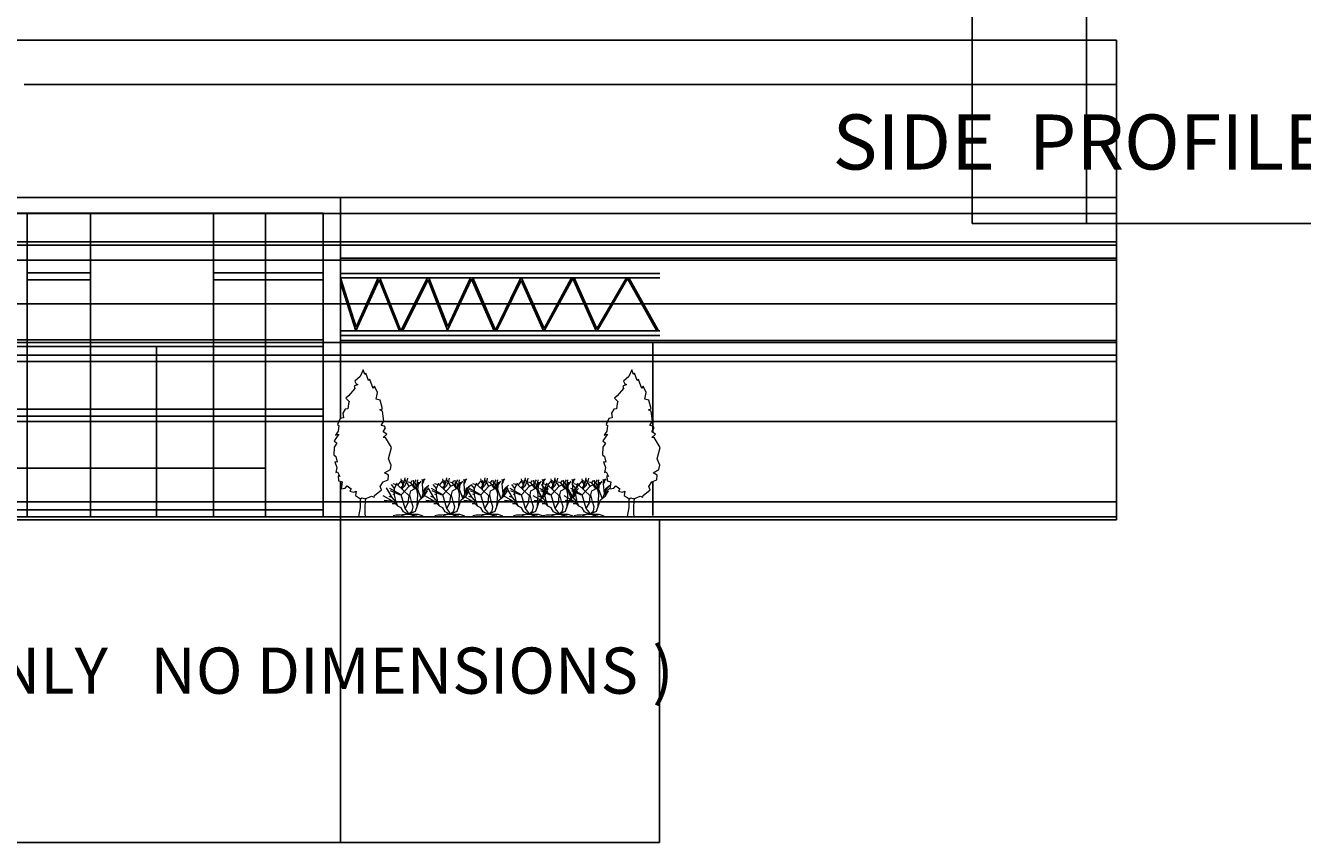
# Model space of a CAD drawing. Units: inches. Extents: x -32109 to 33221, y -19197 to 7608.
# Tile 14 of 25: x -741 to 10957, y -19197 to -11718. Entities that reach past the tile are written whole.
import ezdxf

# ---------------------------------------------------------------- set-up
doc = ezdxf.new("R2010")
doc.units = ezdxf.units.IN
doc.header["$MEASUREMENT"] = 0
for name, color, linetype, lineweight in [('A-ANNO-DIMS', 2, 'Continuous', 18), ('A-ANNO-TEXT', 7, 'Continuous', 25), ('A-ELEV', 7, 'Continuous', 25), ('L-PLNT', 3, 'Continuous', 13)]:
    doc.layers.add(name, color=color, linetype=linetype, lineweight=lineweight)
doc.styles.get("Standard").update_dxf_attribs({"font": 'arial.ttf'})
doc.dimstyles.get("Standard").update_dxf_attribs({"dimtxt": 0.18, "dimasz": 0.18, "dimexe": 0.18, "dimexo": 0.0625, "dimgap": 0.09, "dimtad": 0, "dimtih": 1, "dimtoh": 1, "dimdec": 4, "dimzin": 0, "dimdsep": 46, "dimtxsty": 'Standard', "dimcen": 0.09, "dimadec": 0, "dimazin": 0, "dimtfac": 1, "dimtdec": 4, "dimtofl": 0, "dimtmove": 0, "dimatfit": 3, "dimfxl": 1, "dimtolj": 1, "dimtzin": 0, "dimarcsym": 0})

# ---------------------------------------------------------------- blocks, each defined once
blk = doc.blocks.new('*U2')
blk.add_lwpolyline([(-2.75400000000036, 191.699), (-6.7800000000002, 182.8509999999996), (-13.68200000000024, 176.9529999999995), (-11.95600000000013, 173.2659999999996), (-9.655999999999949, 172.529), (-14.25700000000006, 170.317), (-13.68200000000024, 167.3679999999999), (-21.73300000000017, 157.7829999999999), (-25.1840000000002, 154.8340000000003), (-21.15800000000036, 150.4099999999998), (-21.73300000000017, 147.4609999999998), (-22.88400000000001, 140.8249999999998), (-26.33400000000029, 140.087), (-29.21000000000004, 134.9259999999995), (-28.63499999999977, 129.0279999999998), (-32.66100000000006, 128.2909999999997), (-36.11099999999988, 120.1799999999998), (-34.38599999999997, 118.7059999999997), (-35.53600000000006, 111.3329999999996), (-38.98700000000008, 106.1709999999998), (-34.38599999999997, 107.6459999999997), (-40.71199999999999, 98.79799999999977), (-37.26099999999997, 95.8489999999997), (-40.71199999999999, 90.68799999999965), (-41.28700000000026, 80.36599999999999), (-38.41200000000026, 78.154), (-36.68600000000015, 70.78099999999995), (-39.5619999999999, 71.51799999999957), (-37.26099999999997, 64.14499999999998), (-38.41200000000026, 57.50899999999956), (-36.11099999999988, 58.24699999999984), (-33.23599999999988, 52.3479999999995), (-35.53600000000006, 53.08599999999978), (-34.96100000000024, 46.44999999999981), (-30.36000000000013, 44.9749999999999), (-31.50999999999977, 36.1279999999997), (-26.33400000000029, 36.86499999999978), (-23.45900000000029, 39.81399999999985), (-18.28300000000036, 36.1279999999997), (-20.00800000000027, 33.17799999999988), (-14.83199999999988, 31.70399999999972), (-11.95600000000013, 33.17799999999988), (-12.53099999999995, 27.27999999999975), (-6.204999999999927, 22.85599999999977), (-3.9050000000002, 24.33099999999968), (0.1209999999996398, 22.85599999999977), (8.172999999999774, 26.54299999999967), (11.62399999999979, 25.06799999999976), (12.19900000000007, 27.27999999999975), (21.40000000000009, 34.6529999999998), (19.67500000000018, 39.07699999999977), (23.70099999999957, 44.9749999999999), (30.02700000000004, 47.92399999999997), (30.60199999999986, 53.82299999999986), (25.42599999999993, 56.77199999999993), (32.90299999999979, 61.19599999999991), (34.05299999999988, 67.0939999999996), (30.60199999999986, 75.20499999999993), (34.6279999999997, 89.95100000000002), (26.57599999999957, 103.2219999999997), (23.70099999999957, 103.2219999999997), (28.30199999999968, 107.6459999999997), (23.70099999999957, 110.5949999999998), (26.57599999999957, 115.7559999999994), (25.42599999999993, 117.9679999999998), (20.82499999999982, 118.7059999999997), (24.27599999999984, 124.6040000000002), (22.55099999999993, 137.8759999999997), (19.09999999999991, 139.3499999999999), (22.55099999999993, 140.8249999999998), (19.67500000000018, 151.884), (14.49899999999979, 153.3589999999999), (16.22400000000016, 162.2069999999999), (12.19900000000007, 170.317), (10.47299999999995, 167.3679999999999), (5.871999999999843, 179.1649999999999), (4.146999999999934, 177.69), (0.6959999999999127, 187.2749999999996), (-0.4540000000001783, 185.7999999999997)], close=True)
for points in [[(-6.813000000000101, 23.66899999999987), (-6.813000000000101, 11.66899999999987), (-8.626999999999953, 0)], [(0.3869999999997162, 23.66899999999987), (-0.5760000000000219, 13.27099999999973), (-0.5760000000000219, 3.685999999999694), (0, 0)]]:
    blk.add_lwpolyline(points)
blk = doc.blocks.new('*U3')
for p, q in [((-18.23999999999978, 11.03999999999996), (-21.75499999999988, 16.65499999999997)), ((-12.95999999999981, 12.47999999999979), (-19.67999999999983, 16.31999999999993)), ((-16.79999999999995, 16.31999999999993), (-18.7199999999998, 18.7199999999998)), ((-14.87999999999988, 18.24000000000001), (-17.75999999999999, 19.19999999999982)), ((-16.79999999999995, 16.31999999999993), (-15.3599999999999, 19.67999999999983)), ((-16.79999999999995, 12.47999999999979), (-16.79999999999995, 16.31999999999993)), ((-14.87999999999988, 18.24000000000001), (-12.95999999999981, 20.63999999999987)), ((-8.160000000000082, 12), (-14.87999999999988, 18.24000000000001)), ((-13.32499999999982, 16.72399999999993), (-11.43299999999999, 18.28899999999976)), ((-12.95999999999981, 12.47999999999979), (-8.160000000000082, 17.75999999999999)), ((-12.47099999999977, 19.77499999999986), (-12.89799999999991, 22.04399999999987)), ((-11.67699999999991, 19.07099999999991), (-12.47099999999977, 19.77499999999986)), ((-11.27999999999997, 19.61899999999991), (-12.10400000000004, 21.18399999999974)), ((-12.04299999999989, 15.6279999999997), (-11.92099999999982, 18.83600000000001)), ((-11.98199999999997, 16.80199999999968), (-10.57899999999995, 18.05399999999986)), ((-11.92099999999982, 18.83600000000001), (-10.6400000000001, 20.40100000000007)), ((-11.43299999999999, 18.28899999999976), (-10.45699999999988, 22.7489999999998)), ((-10.57899999999995, 18.05399999999986), (-9.845999999999776, 19.69699999999966)), ((-8.160000000000082, 17.75999999999999), (-10.55999999999994, 21.59999999999991)), ((-9.480000000000018, 19.77499999999986), (-8.991999999999962, 22.59199999999964)), ((-7.200000000000045, 19.67999999999983), (-8.6400000000001, 20.15999999999985)), ((-8.160000000000082, 17.75999999999999), (-5.279999999999972, 19.19999999999982)), ((-7.200000000000045, 19.67999999999983), (-6.240000000000009, 21.11999999999989)), ((-4.799999999999954, 16.31999999999993), (-7.200000000000045, 19.67999999999983)), ((-7.200000000000045, 14.87999999999988), (-3.840000000000145, 16.79999999999995)), ((-5.085999999999785, 17.74099999999998), (-5.512999999999919, 21.33999999999992)), ((-5.279999999999972, 19.19999999999982), (-3.840000000000145, 21.59999999999991)), ((-3.376999999999952, 15.31499999999982), (-5.085999999999785, 17.81899999999973)), ((-2.880000000000109, 12.95999999999981), (-4.319999999999936, 19.67999999999983)), ((-3.840000000000145, 16.79999999999995), (-0.9600000000000363, 20.63999999999987)), ((-3.376999999999952, 18.60199999999963), (-2.887999999999919, 21.57499999999982)), ((-2.765999999999849, 16.80199999999968), (-3.376999999999952, 18.60199999999963)), ((-2.880000000000109, 15.83999999999992), (-2.40000000000009, 20.15999999999985)), ((-0.9600000000000363, 10.55999999999994), (-2.880000000000109, 15.83999999999992)), ((-0.5079999999998109, 21.88799999999969), (-0.0809999999999036, 20.55799999999976)), ((-0.2029999999999745, 19.14899999999988), (0.1020000000000891, 21.33999999999992)), ((0.3460000000000036, 13.20299999999974), (-0.2029999999999745, 19.14899999999988)), ((-0.1419999999998254, 19.38399999999979), (0.5899999999999181, 20.40100000000007)), ((-0.0199999999999818, 20.00999999999999), (0.895999999999958, 21.10499999999979)), ((0.04099999999994, 20.71399999999994), (1.384000000000241, 22.04399999999987)), ((0.1020000000000891, 21.33999999999992), (0.8350000000000363, 21.88799999999969)), ((0.3460000000000036, 13.20299999999974), (1.323000000000092, 16.2539999999999)), ((0.9600000000000363, 12), (1.440000000000054, 15.3599999999999)), ((1.323000000000092, 16.2539999999999), (3.642000000000052, 18.28899999999976)), ((1.440000000000054, 15.3599999999999), (2.879999999999881, 17.27999999999997)), ((1.920000000000072, 13.43999999999982), (2.399999999999863, 15.3599999999999)), ((2.399999999999863, 15.3599999999999), (3.359999999999899, 16.31999999999993)), ((-17.75999999999999, 8.639999999999873), (-23.66300000000001, 11.96100000000001)), ((-17.75999999999999, 8.639999999999873), (-23.12799999999993, 9.221999999999753)), ((-18.23999999999978, 11.03999999999996), (-20.15999999999985, 11.51999999999998)), ((-13.91999999999984, 12.47999999999979), (-19.19999999999982, 14.87999999999988)), ((-15.83999999999992, 8.159999999999854), (-18.23999999999978, 11.03999999999996)), ((-16.79999999999995, 12.47999999999979), (-17.75999999999999, 12.95999999999981)), ((-14.87999999999988, 5.75999999999999), (-17.75999999999999, 8.639999999999873)), ((-15.83999999999992, 8.159999999999854), (-16.79999999999995, 12.47999999999979)), ((-14.87999999999988, 5.75999999999999), (-15.83999999999992, 8.159999999999854)), ((-12.95999999999981, 12.47999999999979), (-13.91999999999984, 12.47999999999979)), ((-10.55999999999994, 4.319999999999936), (-12.95999999999981, 12.47999999999979)), ((-10.55999999999994, 4.319999999999936), (-8.6400000000001, 7.679999999999836)), ((-8.6400000000001, 7.679999999999836), (-8.160000000000082, 12)), ((-7.680000000000063, 12.47999999999979), (-7.200000000000045, 14.87999999999988)), ((-6.720000000000027, 8.639999999999873), (-7.680000000000063, 12.47999999999979)), ((-5.75999999999999, 5.279999999999972), (-6.720000000000027, 8.639999999999873)), ((-4.319999999999936, 2.879999999999881), (-1.920000000000072, 9.599999999999909)), ((-3.360000000000127, 5.279999999999972), (-2.880000000000109, 12.95999999999981)), ((-1.920000000000072, 9.599999999999909), (0.9600000000000363, 12)), ((-0.4800000000000182, 10.79999999999995), (0.3460000000000036, 13.20299999999974)), ((0.9600000000000363, 12), (2.879999999999881, 14.87999999999988)), ((-16.31999999999993, 7.199999999999818), (-18.23999999999978, 7.199999999999818)), ((-15.83999999999992, 0.4799999999997909), (-17.75999999999999, 0)), ((-13.43999999999982, 0.4799999999997909), (-15.83999999999992, 0.4799999999997909)), ((-12.95999999999981, 4.799999999999954), (-14.87999999999988, 5.75999999999999)), ((-9.600000000000136, 0.959999999999809), (-13.43999999999982, 0.4799999999997909)), ((-11.51999999999998, 2.399999999999863), (-12.95999999999981, 4.799999999999954)), ((-9.600000000000136, 0.959999999999809), (-12.95999999999981, 0)), ((-8.6400000000001, 0.959999999999809), (-11.51999999999998, 2.399999999999863)), ((-8.6400000000001, 1.919999999999845), (-10.55999999999994, 4.319999999999936)), ((-9.600000000000136, 0.959999999999809), (-7.680000000000063, 0.959999999999809)), ((-8.6400000000001, 0.959999999999809), (-4.319999999999936, 2.879999999999881)), ((-8.6400000000001, 0.959999999999809), (-6.240000000000009, 2.879999999999881)), ((-8.6400000000001, 0.959999999999809), (-8.6400000000001, 1.919999999999845)), ((-8.6400000000001, 0.959999999999809), (-2.880000000000109, 0.959999999999809)), ((-7.680000000000063, 0.959999999999809), (-6.240000000000009, 0.4799999999997909)), ((-6.240000000000009, 2.879999999999881), (-5.75999999999999, 5.279999999999972)), ((-6.240000000000009, 0.4799999999997909), (-3.360000000000127, 0)), ((-2.880000000000109, 0.959999999999809), (0, 0))]:
    blk.add_line(p, q)
blk = doc.blocks.new('*D13')
at = {"layer": 'A-ANNO-DIMS', "color": 0, "lineweight": -2, "transparency": 16777216}
for p, q in [((-21916.328365, -16214.873241), (-21916.328365, -19197.348741)), ((5067.151383999999, -16244.175331), (5067.151383999999, -19197.348741)), ((-21916.148365, -19197.168741), (-8425.018722423602, -19197.168741)), ((5066.971383999999, -19197.168741), (-8424.158258576399, -19197.168741))]:
    blk.add_line(p, q, dxfattribs=at)
at = {"layer": 'A-ANNO-DIMS', "color": 0, "transparency": 16777216}
for points in [[(-21916.148365, -19197.138741), (-21916.148365, -19197.198741), (-21916.328365, -19197.168741)], [(5066.971383999999, -19197.138741), (5066.971383999999, -19197.198741), (5067.151383999999, -19197.168741)]]:
    blk.add_solid(points, dxfattribs=at)
at = {"layer": 'Defpoints', "color": 0, "transparency": 16777216}
for p in [(-21916.328365, -16214.810741), (5067.151383999999, -16244.112831), (5067.151383999999, -19197.168741)]:
    blk.add_point(p, dxfattribs=at)
at = {"layer": 'A-ANNO-DIMS', "color": 0, "transparency": 16777216, "insert": (-8424.5884905, -19197.168741), "char_height": 0.18, "attachment_point": 5}
blk.add_mtext('\\A1;26983', dxfattribs=at)
blk = doc.blocks.new('*D14')
at = {"layer": 'A-ANNO-DIMS', "color": 0, "lineweight": -2, "transparency": 16777216}
for p, q in [((-18893.90707200001, -10978.730223), (-32108.36667400003, -10978.73022300001)), ((-32108.18667400003, -10978.91022300001), (-32108.18667400003, -13611.23962386222)), ((-32108.18667400003, -16243.93283100001), (-32108.18667400003, -13611.6034301378)), ((5067.088884000002, -16244.11283100001), (-32108.36667400003, -16244.11283100001))]:
    blk.add_line(p, q, dxfattribs=at)
at = {"layer": 'A-ANNO-DIMS', "color": 0, "transparency": 16777216}
for points in [[(-32108.21667400003, -10978.91022300001), (-32108.15667400003, -10978.91022300001), (-32108.18667400003, -10978.73022300001)], [(-32108.21667400003, -16243.93283100001), (-32108.15667400003, -16243.93283100001), (-32108.18667400003, -16244.11283100001)]]:
    blk.add_solid(points, dxfattribs=at)
at = {"layer": 'Defpoints', "color": 0, "transparency": 16777216}
for p in [(-18893.84457200001, -10978.730223), (-32108.18667400003, -16244.11283100001), (5067.151384000002, -16244.11283100001)]:
    blk.add_point(p, dxfattribs=at)
at = {"layer": 'A-ANNO-DIMS', "color": 0, "transparency": 16777216, "insert": (-32108.18667400002, -13611.421527), "char_height": 0.18, "attachment_point": 5}
blk.add_mtext('\\A1;5265', dxfattribs=at)
blk = doc.blocks.new('*D92')
at = {"layer": 'A-ANNO-DIMS', "color": 0, "lineweight": -2, "transparency": 16777216}
for p, q in [((-8664.080497000004, -13437.20315700001), (9252.673715000004, -13437.203157)), ((9252.493715000008, -13437.383157), (9252.493715000008, -14825.82504586221)), ((9252.493715000008, -16214.630741), (9252.493715000008, -14826.18885213779)), ((-8664.080497000004, -16214.810741), (9252.673715000004, -16214.810741))]:
    blk.add_line(p, q, dxfattribs=at)
at = {"layer": 'A-ANNO-DIMS', "color": 0, "transparency": 16777216}
for points in [[(9252.463715000007, -13437.383157), (9252.523715000007, -13437.383157), (9252.493715000008, -13437.203157)], [(9252.463715000007, -16214.630741), (9252.523715000007, -16214.630741), (9252.493715000008, -16214.810741)]]:
    blk.add_solid(points, dxfattribs=at)
at = {"layer": 'Defpoints', "color": 0, "transparency": 16777216}
for p in [(-8664.142997000004, -13437.20315700001), (-8664.142997000004, -16214.810741), (9252.493715000008, -16214.810741)]:
    blk.add_point(p, dxfattribs=at)
at = {"layer": 'A-ANNO-DIMS', "color": 0, "transparency": 16777216, "insert": (9252.493715000002, -14826.006949), "char_height": 0.18, "attachment_point": 5}
blk.add_mtext('\\A1;2777.6', dxfattribs=at)
blk = doc.blocks.new('*D99')
at = {"layer": 'A-ANNO-DIMS', "color": 0, "lineweight": -2, "transparency": 16777216}
for p, q in [((-9175.094027000003, -13729.028041), (9252.67371500001, -13729.028041)), ((9252.493715000008, -13729.208041), (9252.493715000008, -13997.52187397067)), ((9252.493715000008, -14266.199636), (9252.493715000008, -13997.88580302933)), ((-9175.094027000003, -14266.37963600001), (9252.67371500001, -14266.379636))]:
    blk.add_line(p, q, dxfattribs=at)
at = {"layer": 'A-ANNO-DIMS', "color": 0, "transparency": 16777216}
for points in [[(9252.463715000007, -13729.208041), (9252.523715000007, -13729.208041), (9252.493715000008, -13729.028041)], [(9252.463715000007, -14266.199636), (9252.523715000007, -14266.199636), (9252.493715000008, -14266.379636)]]:
    blk.add_solid(points, dxfattribs=at)
at = {"layer": 'Defpoints', "color": 0, "transparency": 16777216}
for p in [(-9175.156527000003, -13729.028041), (-9175.156527000003, -14266.37963600001), (9252.493715000008, -14266.379636)]:
    blk.add_point(p, dxfattribs=at)
at = {"layer": 'A-ANNO-DIMS', "color": 0, "transparency": 16777216, "insert": (9252.493715000002, -13997.7038385), "char_height": 0.18, "attachment_point": 5}
blk.add_mtext('\\A1;537.4', dxfattribs=at)
blk = doc.blocks.new('*D100')
at = {"layer": 'A-ANNO-DIMS', "color": 0, "lineweight": -2, "transparency": 16777216}
for p, q in [((-9175.094027000003, -14266.37963600001), (9252.67371500001, -14266.379636)), ((9252.493715000008, -14266.559636), (9252.493715000008, -14530.56642486221)), ((9252.493715000008, -14794.93702), (9252.493715000008, -14530.93023113779)), ((-9175.094027000003, -14795.11702), (9252.67371500001, -14795.11702))]:
    blk.add_line(p, q, dxfattribs=at)
at = {"layer": 'A-ANNO-DIMS', "color": 0, "transparency": 16777216}
for points in [[(9252.463715000007, -14266.559636), (9252.523715000007, -14266.559636), (9252.493715000008, -14266.379636)], [(9252.463715000007, -14794.93702), (9252.523715000007, -14794.93702), (9252.493715000008, -14795.11702)]]:
    blk.add_solid(points, dxfattribs=at)
at = {"layer": 'Defpoints', "color": 0, "transparency": 16777216}
for p in [(-9175.156527000003, -14266.37963600001), (-9175.156527000003, -14795.11702), (9252.493715000008, -14795.11702)]:
    blk.add_point(p, dxfattribs=at)
at = {"layer": 'A-ANNO-DIMS', "color": 0, "transparency": 16777216, "insert": (9252.493715000002, -14530.748328), "char_height": 0.18, "attachment_point": 5}
blk.add_mtext('\\A1;528.7', dxfattribs=at)
blk = doc.blocks.new('*D101')
at = {"layer": 'A-ANNO-DIMS', "color": 0, "lineweight": -2, "transparency": 16777216}
for p, q in [((-9175.094027000003, -14795.11702), (9252.67371500001, -14795.11702)), ((9252.493715000008, -14795.29702), (9252.493715000008, -15068.37273186222)), ((9252.493715000008, -15341.81225), (9252.493715000008, -15068.73653813779)), ((-9175.094027000003, -15341.99225), (9252.67371500001, -15341.99225))]:
    blk.add_line(p, q, dxfattribs=at)
at = {"layer": 'A-ANNO-DIMS', "color": 0, "transparency": 16777216}
for points in [[(9252.463715000007, -14795.29702), (9252.523715000007, -14795.29702), (9252.493715000008, -14795.11702)], [(9252.463715000007, -15341.81225), (9252.523715000007, -15341.81225), (9252.493715000008, -15341.99225)]]:
    blk.add_solid(points, dxfattribs=at)
at = {"layer": 'Defpoints', "color": 0, "transparency": 16777216}
for p in [(-9175.156527000003, -14795.11702), (-9175.156527000003, -15341.99225), (9252.493715000008, -15341.99225)]:
    blk.add_point(p, dxfattribs=at)
at = {"layer": 'A-ANNO-DIMS', "color": 0, "transparency": 16777216, "insert": (9252.493715, -15068.554635), "char_height": 0.18, "attachment_point": 5}
blk.add_mtext('\\A1;546.9', dxfattribs=at)
blk = doc.blocks.new('*D102')
at = {"layer": 'A-ANNO-DIMS', "color": 0, "lineweight": -2, "transparency": 16777216}
for p, q in [((-9175.094027000003, -15341.99225), (9252.67371500001, -15341.99225)), ((9252.493715000008, -15342.17225), (9252.493715000008, -15710.46428297067)), ((9252.493715000008, -16079.120245), (9252.493715000008, -15710.82821202933)), ((-9175.094027000003, -16079.300245), (9252.67371500001, -16079.300245))]:
    blk.add_line(p, q, dxfattribs=at)
at = {"layer": 'A-ANNO-DIMS', "color": 0, "transparency": 16777216}
for points in [[(9252.463715000007, -15342.17225), (9252.523715000007, -15342.17225), (9252.493715000008, -15341.99225)], [(9252.463715000007, -16079.120245), (9252.523715000007, -16079.120245), (9252.493715000008, -16079.300245)]]:
    blk.add_solid(points, dxfattribs=at)
at = {"layer": 'Defpoints', "color": 0, "transparency": 16777216}
for p in [(-9175.156527000003, -15341.99225), (-9175.156527000003, -16079.300245), (9252.493715000008, -16079.300245)]:
    blk.add_point(p, dxfattribs=at)
at = {"layer": 'A-ANNO-DIMS', "color": 0, "transparency": 16777216, "insert": (9252.493715, -15710.6462475), "char_height": 0.18, "attachment_point": 5}
blk.add_mtext('\\A1;737.3', dxfattribs=at)
blk = doc.blocks.new('*D106')
at = {"layer": 'A-ANNO-DIMS', "color": 0, "lineweight": -2, "transparency": 16777216}
for p, q in [((-1331.314498, -16214.873241), (-1331.314498, -19197.348741)), ((2144.247723, -16214.873241), (2144.247723, -19197.348741)), ((-1331.134498, -19197.168741), (406.0031063608458, -19197.168741)), ((2144.067723, -19197.168741), (406.9301186391541, -19197.168741))]:
    blk.add_line(p, q, dxfattribs=at)
at = {"layer": 'A-ANNO-DIMS', "color": 0, "transparency": 16777216}
for points in [[(-1331.134498, -19197.138741), (-1331.134498, -19197.198741), (-1331.314498, -19197.168741)], [(2144.067723, -19197.138741), (2144.067723, -19197.198741), (2144.247723, -19197.168741)]]:
    blk.add_solid(points, dxfattribs=at)
at = {"layer": 'Defpoints', "color": 0, "transparency": 16777216}
for p in [(-1331.314498, -16214.810741), (2144.247723, -16214.810741), (2144.247723, -19197.168741)]:
    blk.add_point(p, dxfattribs=at)
at = {"layer": 'A-ANNO-DIMS', "color": 0, "transparency": 16777216, "insert": (406.4666125, -19197.168741), "char_height": 0.18, "attachment_point": 5}
blk.add_mtext('\\A1;3475.6', dxfattribs=at)
blk = doc.blocks.new('*D107')
at = {"layer": 'A-ANNO-DIMS', "color": 0, "lineweight": -2, "transparency": 16777216}
for p, q in [((2144.247723, -16214.873241), (2144.247723, -19197.348741)), ((5067.151383999999, -16244.175331), (5067.151383999999, -19197.348741)), ((2144.427723, -19197.168741), (3605.339246542292, -19197.168741)), ((5066.971383999999, -19197.168741), (3606.059860457707, -19197.168741))]:
    blk.add_line(p, q, dxfattribs=at)
at = {"layer": 'A-ANNO-DIMS', "color": 0, "transparency": 16777216}
for points in [[(2144.427723, -19197.138741), (2144.427723, -19197.198741), (2144.247723, -19197.168741)], [(5066.971383999999, -19197.138741), (5066.971383999999, -19197.198741), (5067.151383999999, -19197.168741)]]:
    blk.add_solid(points, dxfattribs=at)
at = {"layer": 'Defpoints', "color": 0, "transparency": 16777216}
for p in [(2144.247723, -16214.810741), (5067.151383999999, -16244.112831), (5067.151383999999, -19197.168741)]:
    blk.add_point(p, dxfattribs=at)
at = {"layer": 'A-ANNO-DIMS', "color": 0, "transparency": 16777216, "insert": (3605.6995535, -19197.168741), "char_height": 0.18, "attachment_point": 5}
blk.add_mtext('\\A1;2923', dxfattribs=at)
blk = doc.blocks.new('*D110')
at = {"layer": 'A-ANNO-DIMS', "color": 0, "lineweight": -2, "transparency": 16777216}
for p, q in [((-6449.892839000003, -11850.794233), (9252.67371500001, -11850.794233)), ((9252.493715000004, -11850.974233), (9252.493715000008, -14032.62052247067)), ((9252.493715000008, -16214.630741), (9252.493715000008, -14032.98445152933)), ((-6952.711375000004, -16214.810741), (9252.673715000004, -16214.810741))]:
    blk.add_line(p, q, dxfattribs=at)
at = {"layer": 'A-ANNO-DIMS', "color": 0, "transparency": 16777216}
for points in [[(9252.463715000005, -11850.974233), (9252.523715000007, -11850.974233), (9252.493715000004, -11850.794233)], [(9252.463715000007, -16214.630741), (9252.523715000007, -16214.630741), (9252.493715000008, -16214.810741)]]:
    blk.add_solid(points, dxfattribs=at)
at = {"layer": 'Defpoints', "color": 0, "transparency": 16777216}
for p in [(-6449.955339000005, -11850.794233), (-6952.773875000004, -16214.810741), (9252.493715000008, -16214.810741)]:
    blk.add_point(p, dxfattribs=at)
at = {"layer": 'A-ANNO-DIMS', "color": 0, "transparency": 16777216, "insert": (9252.493715000002, -14032.802487), "char_height": 0.18, "attachment_point": 5}
blk.add_mtext('\\A1;4364', dxfattribs=at)
blk = doc.blocks.new('*D111')
at = {"layer": 'A-ANNO-DIMS', "color": 0, "lineweight": -2, "transparency": 16777216}
for p, q in [((-6954.560451000005, -13699.45890900001), (9252.67371500001, -13699.458909)), ((9252.493715000008, -13699.638909), (9252.493715000008, -14956.95292186222)), ((9252.493715000008, -16214.630741), (9252.493715000008, -14957.31672813779)), ((-6952.711375000004, -16214.810741), (9252.673715000004, -16214.810741))]:
    blk.add_line(p, q, dxfattribs=at)
at = {"layer": 'A-ANNO-DIMS', "color": 0, "transparency": 16777216}
for points in [[(9252.463715000007, -13699.638909), (9252.523715000007, -13699.638909), (9252.493715000008, -13699.458909)], [(9252.463715000007, -16214.630741), (9252.523715000007, -16214.630741), (9252.493715000008, -16214.810741)]]:
    blk.add_solid(points, dxfattribs=at)
at = {"layer": 'Defpoints', "color": 0, "transparency": 16777216}
for p in [(-6954.622951000004, -13699.45890900001), (-6952.773875000004, -16214.810741), (9252.493715000008, -16214.810741)]:
    blk.add_point(p, dxfattribs=at)
at = {"layer": 'A-ANNO-DIMS', "color": 0, "transparency": 16777216, "insert": (9252.493715, -14957.134825), "char_height": 0.18, "attachment_point": 5}
blk.add_mtext('\\A1;2515.4', dxfattribs=at)
blk = doc.blocks.new('*D112')
at = {"layer": 'A-ANNO-DIMS', "color": 0, "lineweight": -2, "transparency": 16777216}
for p, q in [((-754.1744190000001, -12255.931551), (9252.673715000004, -12255.931551)), ((9252.493715000004, -12256.111551), (9252.493715000008, -14235.18918147067)), ((9252.493715000008, -16214.630741), (9252.493715000008, -14235.55311052933)), ((-1331.251998, -16214.810741), (9252.67371500001, -16214.810741))]:
    blk.add_line(p, q, dxfattribs=at)
at = {"layer": 'A-ANNO-DIMS', "color": 0, "transparency": 16777216}
for points in [[(9252.463715000005, -12256.111551), (9252.523715000007, -12256.111551), (9252.493715000004, -12255.931551)], [(9252.463715000007, -16214.630741), (9252.523715000007, -16214.630741), (9252.493715000008, -16214.810741)]]:
    blk.add_solid(points, dxfattribs=at)
at = {"layer": 'Defpoints', "color": 0, "transparency": 16777216}
for p in [(-754.2369190000002, -12255.931551), (-1331.314498, -16214.810741), (9252.493715000008, -16214.810741)]:
    blk.add_point(p, dxfattribs=at)
at = {"layer": 'A-ANNO-DIMS', "color": 0, "transparency": 16777216, "insert": (9252.493715000002, -14235.371146), "char_height": 0.18, "attachment_point": 5}
blk.add_mtext('\\A1;3959', dxfattribs=at)
blk = doc.blocks.new('*D113')
at = {"layer": 'A-ANNO-DIMS', "color": 0, "lineweight": -2, "transparency": 16777216}
for p, q in [((2144.310223000001, -13292.13755), (9252.67371500001, -13292.13755)), ((9252.493715000008, -13292.31755), (9252.493715000008, -14753.29224236221)), ((9252.493715000008, -16214.630741), (9252.493715000008, -14753.65604863779)), ((2144.310223000001, -16214.810741), (9252.67371500001, -16214.810741))]:
    blk.add_line(p, q, dxfattribs=at)
at = {"layer": 'A-ANNO-DIMS', "color": 0, "transparency": 16777216}
for points in [[(9252.463715000007, -13292.31755), (9252.523715000007, -13292.31755), (9252.493715000008, -13292.13755)], [(9252.463715000007, -16214.630741), (9252.523715000007, -16214.630741), (9252.493715000008, -16214.810741)]]:
    blk.add_solid(points, dxfattribs=at)
at = {"layer": 'Defpoints', "color": 0, "transparency": 16777216}
for p in [(2144.247723000001, -13292.13755), (2144.247723000001, -16214.810741), (9252.493715000008, -16214.810741)]:
    blk.add_point(p, dxfattribs=at)
at = {"layer": 'A-ANNO-DIMS', "color": 0, "transparency": 16777216, "insert": (9252.493715000002, -14753.4741455), "char_height": 0.18, "attachment_point": 5}
blk.add_mtext('\\A1;2922.7', dxfattribs=at)
blk = doc.blocks.new('*D114')
at = {"layer": 'A-ANNO-DIMS', "color": 0, "lineweight": -2, "transparency": 16777216}
for p, q in [((-2554.258149000001, -14734.482938), (9252.67371500001, -14734.482938)), ((9252.493715000008, -14734.662938), (9252.493715000008, -15474.46487497067)), ((9252.493715000008, -16214.630741), (9252.493715000008, -15474.82880402933)), ((-2554.258149000001, -16214.810741), (9252.673715000004, -16214.810741))]:
    blk.add_line(p, q, dxfattribs=at)
at = {"layer": 'A-ANNO-DIMS', "color": 0, "transparency": 16777216}
for points in [[(9252.463715000007, -14734.662938), (9252.523715000007, -14734.662938), (9252.493715000008, -14734.482938)], [(9252.463715000007, -16214.630741), (9252.523715000007, -16214.630741), (9252.493715000008, -16214.810741)]]:
    blk.add_solid(points, dxfattribs=at)
at = {"layer": 'Defpoints', "color": 0, "transparency": 16777216}
for p in [(-2554.320649000001, -14734.482938), (-2554.320649000001, -16214.810741), (9252.493715000008, -16214.810741)]:
    blk.add_point(p, dxfattribs=at)
at = {"layer": 'A-ANNO-DIMS', "color": 0, "transparency": 16777216, "insert": (9252.493715, -15474.6468395), "char_height": 0.18, "attachment_point": 5}
blk.add_mtext('\\A1;1480.3', dxfattribs=at)
blk = doc.blocks.new('*D115')
at = {"layer": 'A-ANNO-DIMS', "color": 0, "lineweight": -2, "transparency": 16777216}
for p, q in [((-1331.251998, -13865.04756300001), (9252.67371500001, -13865.047563)), ((9252.493715000008, -13865.227563), (9252.493715000008, -14242.40669386222)), ((9252.493715000008, -14619.949631), (9252.493715000008, -14242.77050013779)), ((-1331.251998, -14620.129631), (9252.67371500001, -14620.129631))]:
    blk.add_line(p, q, dxfattribs=at)
at = {"layer": 'A-ANNO-DIMS', "color": 0, "transparency": 16777216}
for points in [[(9252.463715000007, -13865.227563), (9252.523715000007, -13865.227563), (9252.493715000008, -13865.047563)], [(9252.463715000007, -14619.949631), (9252.523715000007, -14619.949631), (9252.493715000008, -14620.129631)]]:
    blk.add_solid(points, dxfattribs=at)
at = {"layer": 'Defpoints', "color": 0, "transparency": 16777216}
for p in [(-1331.314498, -13865.04756300001), (-1331.314498, -14620.129631), (9252.493715000008, -14620.129631)]:
    blk.add_point(p, dxfattribs=at)
at = {"layer": 'A-ANNO-DIMS', "color": 0, "transparency": 16777216, "insert": (9252.493715000002, -14242.588597), "char_height": 0.18, "attachment_point": 5}
blk.add_mtext('\\A1;755.1', dxfattribs=at)
blk = doc.blocks.new('*D116')
at = {"layer": 'A-ANNO-DIMS', "color": 0, "lineweight": -2, "transparency": 16777216}
for p, q in [((5071.470246000002, -13847.28216900001), (9252.67371500001, -13847.28216900001)), ((9252.493715000008, -13847.46216900001), (9252.493715000008, -14224.64129986222)), ((9252.493715000008, -14602.184237), (9252.493715000008, -14225.0051061378)), ((5071.470246000002, -14602.364237), (9252.67371500001, -14602.364237))]:
    blk.add_line(p, q, dxfattribs=at)
at = {"layer": 'A-ANNO-DIMS', "color": 0, "transparency": 16777216}
for points in [[(9252.463715000007, -13847.46216900001), (9252.523715000007, -13847.46216900001), (9252.493715000008, -13847.28216900001)], [(9252.463715000007, -14602.184237), (9252.523715000007, -14602.184237), (9252.493715000008, -14602.364237)]]:
    blk.add_solid(points, dxfattribs=at)
at = {"layer": 'Defpoints', "color": 0, "transparency": 16777216}
for p in [(5071.407746000001, -13847.28216900001), (5071.407746000001, -14602.364237), (9252.493715000008, -14602.364237)]:
    blk.add_point(p, dxfattribs=at)
at = {"layer": 'A-ANNO-DIMS', "color": 0, "transparency": 16777216, "insert": (9252.493715000002, -14224.823203), "char_height": 0.18, "attachment_point": 5}
blk.add_mtext('\\A1;755.1', dxfattribs=at)
blk = doc.blocks.new('*D117')
at = {"layer": 'A-ANNO-DIMS', "color": 0, "lineweight": -2, "transparency": 16777216}
for p, q in [((5071.470246000002, -14602.364237), (9252.67371500001, -14602.364237)), ((9252.493715000008, -14602.54423700001), (9252.493715000008, -15423.05663086222)), ((9252.493715000008, -16243.932831), (9252.493715000008, -15423.42043713779)), ((5067.213884000001, -16244.11283100001), (9252.67371500001, -16244.11283100001))]:
    blk.add_line(p, q, dxfattribs=at)
at = {"layer": 'A-ANNO-DIMS', "color": 0, "transparency": 16777216}
for points in [[(9252.463715000007, -14602.54423700001), (9252.523715000007, -14602.54423700001), (9252.493715000008, -14602.364237)], [(9252.463715000007, -16243.932831), (9252.523715000007, -16243.932831), (9252.493715000008, -16244.11283100001)]]:
    blk.add_solid(points, dxfattribs=at)
at = {"layer": 'Defpoints', "color": 0, "transparency": 16777216}
for p in [(5071.407746000001, -14602.364237), (5067.151384000002, -16244.11283100001), (9252.493715000008, -16244.11283100001)]:
    blk.add_point(p, dxfattribs=at)
at = {"layer": 'A-ANNO-DIMS', "color": 0, "transparency": 16777216, "insert": (9252.493715, -15423.238534), "char_height": 0.18, "attachment_point": 5}
blk.add_mtext('\\A1;1641.7', dxfattribs=at)
blk = doc.blocks.new('*D118')
at = {"layer": 'A-ANNO-DIMS', "color": 0, "lineweight": -2, "transparency": 16777216}
for p, q in [((7931.85712, -8929.127357), (7931.85712, -13529.670166)), ((8978.112405, -11575.866047), (8978.112405, -13529.670166)), ((7932.03712, -13529.490166), (8454.529605610505, -13529.490166)), ((8977.932405, -13529.490166), (8455.439919389495, -13529.490166))]:
    blk.add_line(p, q, dxfattribs=at)
at = {"layer": 'A-ANNO-DIMS', "color": 0, "transparency": 16777216}
for points in [[(7932.03712, -13529.460166), (7932.03712, -13529.520166), (7931.85712, -13529.490166)], [(8977.932405, -13529.460166), (8977.932405, -13529.520166), (8978.112405, -13529.490166)]]:
    blk.add_solid(points, dxfattribs=at)
at = {"layer": 'Defpoints', "color": 0, "transparency": 16777216}
for p in [(7931.85712, -8929.064857), (8978.112405, -11575.803547), (8978.112405, -13529.490166)]:
    blk.add_point(p, dxfattribs=at)
at = {"layer": 'A-ANNO-DIMS', "color": 0, "transparency": 16777216, "insert": (8454.9847625, -13529.490166), "char_height": 0.18, "attachment_point": 5}
blk.add_mtext('\\A1;1046.3', dxfattribs=at)
blk = doc.blocks.new('*D119')
at = {"layer": 'A-ANNO-DIMS', "color": 0, "lineweight": -2, "transparency": 16777216}
for p, q in [((8978.112405, -11575.866047), (8978.112405, -13529.670166)), ((11053.824937, -11575.866047), (11053.824937, -13529.670166)), ((8978.292405, -13529.490166), (10015.50350728922, -13529.490166)), ((11053.644937, -13529.490166), (10016.43383471078, -13529.490166))]:
    blk.add_line(p, q, dxfattribs=at)
at = {"layer": 'A-ANNO-DIMS', "color": 0, "transparency": 16777216}
for points in [[(8978.292405, -13529.460166), (8978.292405, -13529.520166), (8978.112405, -13529.490166)], [(11053.644937, -13529.460166), (11053.644937, -13529.520166), (11053.824937, -13529.490166)]]:
    blk.add_solid(points, dxfattribs=at)
at = {"layer": 'Defpoints', "color": 0, "transparency": 16777216}
for p in [(8978.112405, -11575.803547), (11053.824937, -11575.803547), (11053.824937, -13529.490166)]:
    blk.add_point(p, dxfattribs=at)
at = {"layer": 'A-ANNO-DIMS', "color": 0, "transparency": 16777216, "insert": (10015.968671, -13529.490166), "char_height": 0.18, "attachment_point": 5}
blk.add_mtext('\\A1;2075.7', dxfattribs=at)

msp = doc.modelspace()

# ---------------------------------------------------------------- linework, layer by layer
at = {"layer": 'A-ELEV'}
for p, q in [((-1331.314497847143, -13292.13755024582), (2144.247722834968, -13292.13755024587)), ((2144.247722834968, -13292.13755024587), (2144.247722834968, -15313.80774676814)), ((-1195.361884540551, -13434.77154261943), (1987.069161839619, -13434.77154261943)), ((-727.0279749792153, -16214.81074108689), (-727.0279749792153, -13434.77154261943)), ((-144.1667642799402, -16214.81074108689), (-144.1667642799402, -13434.77154261943)), ((982.0397144143125, -16214.81074108689), (982.0397144143125, -13434.77154261943)), ((1456.231965364462, -16214.81074108689), (1456.231965364462, -13434.77154261943)), ((1987.069161839619, -13434.77154261943), (1987.069161839619, -16214.81074108689)), ((5071.407746090578, -13847.28216883123), (2144.247722834968, -13847.28216883123)), ((-727.0279749792153, -13980.77708959707), (-144.1667642799402, -13980.77708959707)), ((982.0397144143125, -13980.77708959707), (1987.069161839619, -13980.77708959707)), ((5071.407746090578, -13987.17885652265), (2144.247722834968, -13987.17885652265)), ((5071.407746090578, -14028.99827845845), (2144.247722834949, -14028.99827845845)), ((2287.614096013806, -14480.74364340453), (2144.247722834949, -14028.99827845845)), ((2490.620416074603, -14028.99827845845), (2287.614096013806, -14480.74364340453)), ((2697.632563547125, -14514.09204573893), (2504.78405839074, -14028.65800699722)), ((2940.686911448869, -14028.99827845845), (2697.632563547125, -14514.09204573893)), ((3126.892712163601, -14473.87319611016), (2954.393621457929, -14028.99827845845)), ((3336.648858452214, -14028.99827845845), (3126.892712163601, -14473.87319611016)), ((3563.969595058387, -14506.26875214773), (3355.60805916634, -14028.99827845845)), ((3795.985597446974, -14028.99827845845), (3563.969595058387, -14506.26875214773)), ((4009.686502914906, -14491.56795467733), (3803.556154595047, -14028.99827845845)), ((4261.326152075516, -14028.99827845845), (4009.686502914906, -14491.56795467733)), ((4272.627065814413, -14034.96762397618), (4011.981572616114, -14514.09204573893)), ((4488.15992611747, -14513.44262639094), (4272.627065814413, -14034.96762397618)), ((4493.358515028083, -14493.86747508671), (4283.954497868559, -14028.99827845845)), ((4763.621111903307, -14028.99827845845), (4493.358515028083, -14493.86747508671)), ((4774.994375510096, -14034.86226691171), (4496.38291778139, -14514.09204573893)), ((5042.295209871197, -14514.09204573893), (4774.994375510096, -14034.86226691171)), ((5056.928367454137, -14514.09204573893), (4786.356765967343, -14028.99827845845)), ((-727.0279749792153, -14046.11463650732), (-144.1667642799402, -14046.11463650732)), ((982.0397144143125, -14046.11463650732), (1987.069161839619, -14046.11463650732)), ((2284.789806687225, -14514.09204573893), (2144.247722834968, -14071.24597554564)), ((2497.485274710293, -14044.89982496818), (2286.638648422941, -14514.09204573893)), ((2683.881388672956, -14514.09204573893), (2497.485274710293, -14044.89982496818)), ((2946.922873434335, -14045.0808158412), (2711.926618420664, -14514.09204573893)), ((3125.747294638481, -14506.26875214773), (2946.922873434335, -14045.0808158412)), ((3346.045438429631, -14039.0351558408), (3125.747294638481, -14506.26875214773)), ((3553.440592062612, -14514.09204573893), (3346.045438429631, -14039.0351558408)), ((3799.431692020136, -14051.13962576468), (3574.376140294388, -14514.09204573893)), ((4004.564390801782, -14511.47051265617), (3799.431692020136, -14051.13962576468)), ((-1195.361884540551, -14595.055217791), (1987.069161839619, -14595.055217791)), ((2165.401344110982, -14514.09204573893), (2144.247722834968, -14514.09204573893)), ((2165.401344110982, -14555.29605210392), (2144.247722834968, -14555.29605210392)), ((5071.407746090578, -14602.36423700717), (2144.247722834968, -14602.36423700717)), ((5071.407746090578, -14514.09204573893), (2165.401344110982, -14514.09204573893)), ((2165.401344110982, -14555.29605210392), (5071.407746090578, -14555.29605210392)), ((5005.787831488589, -15442.77112314417), (5005.787831488589, -14613.24698265352)), ((-1195.361884540551, -14656.76288104973), (1987.069161839619, -14656.76288104973)), ((458.4526523961021, -16214.81074108689), (458.4526523961021, -14656.76288104973)), ((-1195.361884540551, -15231.59175844843), (1987.069161839619, -15231.59175844843)), ((-1195.361884540551, -15293.29942170716), (1987.069161839619, -15293.29942170716)), ((5005.787831488589, -15489.48455487615), (5005.787831488589, -15482.18204576999)), ((-1195.361884540551, -15769.95997281254), (1456.231965364462, -15769.95997281254)), ((2144.247722834968, -15892.33437797295), (2144.247722834968, -16214.81074108689)), ((5005.787831488589, -16203.76688847666), (5005.787831488589, -15893.43787873083)), ((-12087.2256698305, -16214.81074108689), (7362.493715378476, -16214.81074108689)), ((-1195.361884540551, -16151.09533420663), (1987.069161839619, -16151.09533420663))]:
    msp.add_line(p, q, dxfattribs=at)

# ---------------------------------------------------------------- block references
at = {"layer": 'L-PLNT'}
for name, p, xscale, yscale, zscale in [('*U2', (2371.130985600996, -16211.62164771251), 6.995961062916478, 6.995961062916478, 6.995961062916478), ('*U2', (4832.381882839708, -16211.62164771251), 6.995961062916478, 6.995961062916478, 6.995961062916478), ('*U3', (2898.068777348983, -16206.68344137856), 15.30854395898754, 15.30854395898754, 15.30854395898754), ('*U3', (3279.98716565301, -16206.68344137856), 15.30854395898754, 15.30854395898754, 15.30854395898754), ('*U3', (3629.169558031207, -16206.68344137856), 15.30854395898754, 15.30854395898754, 15.30854395898754), ('*U3', (4000.175791276901, -16206.68344137856), 15.30854395898754, 15.30854395898754, 15.30854395898754), ('*U3', (4272.97474061889, -16206.68344137856), 15.30854395898754, 15.30854395898754, 15.30854395898754), ('*U3', (4556.685375770045, -16206.68344137856), 15.30854395898754, 15.30854395898754, 15.30854395898754)]:
    msp.add_blockref(name, p, dxfattribs=dict(at, xscale=xscale, yscale=yscale, zscale=zscale))

# ---------------------------------------------------------------- texts
at = {"layer": 'A-ANNO-TEXT'}
for s, height, p in [('SIDE  PROFILE   ATRIUM   CIRCULATION   AND   VERTICAL   CIRCULATION   HUB', 504.218310670369, (6653.0921668488, -13035.81166412015)), ('  ( CONCEPTUAL ONLY   NO DIMENSIONS )', 423.0385369056507, (-5876.466612907216, -17835.72336381357))]:
    msp.add_text(s, height=height, dxfattribs=at).set_placement(p)

# ---------------------------------------------------------------- dimensions: what is measured, and where the dimension line sits
at = {"layer": 'A-ANNO-DIMS'}
for base, p1, p2, override, picture, middle in [((8978.112405, -13529.490166), (7931.85712, -8929.064857), (8978.112405, -11575.803547), {"dimdec": 1, "dimlfac": 1, "dimrnd": 0, "dimzin": 0, "dimdsep": 46, "dimlunit": 2}, '*D118', (8454.9847625, -13529.490166)), ((11053.824937, -13529.490166), (8978.112405, -11575.803547), (11053.824937, -11575.803547), {"dimdec": 1, "dimlfac": 1, "dimrnd": 0, "dimzin": 0, "dimdsep": 46, "dimlunit": 2}, '*D119', (10015.968671, -13529.490166)), ((5067.151383999999, -19197.168741), (-21916.328365, -16214.810741), (5067.151383999999, -16244.112831), {"dimdec": 0, "dimlfac": 1, "dimrnd": 0, "dimzin": 0, "dimdsep": 46, "dimlunit": 2}, '*D13', (-8424.5884905, -19197.168741)), ((2144.247723, -19197.168741), (-1331.314498, -16214.810741), (2144.247723, -16214.810741), {"dimdec": 1, "dimlfac": 1, "dimrnd": 0, "dimzin": 0, "dimdsep": 46, "dimlunit": 2}, '*D106', (406.4666125, -19197.168741)), ((5067.151383999999, -19197.168741), (2144.247723, -16214.810741), (5067.151383999999, -16244.112831), {"dimdec": 0, "dimlfac": 1, "dimrnd": 0, "dimzin": 0, "dimdsep": 46, "dimlunit": 2}, '*D107', (3605.6995535, -19197.168741))]:
    dim = msp.add_linear_dim(base=base, p1=p1, p2=p2, dimstyle='Standard', override=override, dxfattribs=at)
    dim.commit()
    dim.dimension.update_dxf_attribs({"geometry": picture, "text_midpoint": middle})
for base, p1, p2, override, picture, middle in [((-32108.18667400003, -16244.11283100001), (-18893.844572, -10978.730223), (5067.151383999999, -16244.112831), {"dimdec": 0, "dimlfac": 1, "dimrnd": 0, "dimzin": 0, "dimdsep": 46, "dimlunit": 2}, '*D14', (-32108.18667400002, -13611.421527)), ((9252.493715000008, -16214.810741), (-6449.955339, -11850.794233), (-6952.773875, -16214.810741), {"dimdec": 0, "dimlfac": 1, "dimrnd": 0, "dimzin": 0, "dimdsep": 46, "dimlunit": 2}, '*D110', (9252.493715000002, -14032.802487)), ((9252.493715000008, -16214.810741), (-754.236919, -12255.931551), (-1331.314498, -16214.810741), {"dimdec": 0, "dimlfac": 1, "dimrnd": 0, "dimzin": 0, "dimdsep": 46, "dimlunit": 2}, '*D112', (9252.493715000002, -14235.371146)), ((9252.493715000008, -16214.810741), (2144.247723, -13292.13755), (2144.247723, -16214.810741), {"dimdec": 1, "dimlfac": 1, "dimrnd": 0, "dimzin": 0, "dimdsep": 46, "dimlunit": 2}, '*D113', (9252.493715000002, -14753.4741455)), ((9252.493715000008, -16214.810741), (-8664.142997, -13437.203157), (-8664.142997, -16214.810741), {"dimdec": 1, "dimlfac": 1, "dimrnd": 0, "dimzin": 0, "dimdsep": 46, "dimlunit": 2}, '*D92', (9252.493715000002, -14826.006949)), ((9252.493715000008, -14266.379636), (-9175.156527, -13729.028041), (-9175.156527, -14266.379636), {"dimdec": 1, "dimlfac": 1, "dimrnd": 0, "dimzin": 0, "dimdsep": 46, "dimlunit": 2}, '*D99', (9252.493715000002, -13997.7038385)), ((9252.493715000008, -16214.810741), (-6954.622951000001, -13699.458909), (-6952.773875, -16214.810741), {"dimdec": 1, "dimlfac": 1, "dimrnd": 0, "dimzin": 0, "dimdsep": 46, "dimlunit": 2}, '*D111', (9252.493715, -14957.134825)), ((9252.493715000008, -14620.129631), (-1331.314498, -13865.047563), (-1331.314498, -14620.129631), {"dimdec": 1, "dimlfac": 1, "dimrnd": 0, "dimzin": 0, "dimdsep": 46, "dimlunit": 2}, '*D115', (9252.493715000002, -14242.588597)), ((9252.493715000008, -14602.364237), (5071.407746, -13847.282169), (5071.407746, -14602.364237), {"dimdec": 1, "dimlfac": 1, "dimrnd": 0, "dimzin": 0, "dimdsep": 46, "dimlunit": 2}, '*D116', (9252.493715000002, -14224.823203)), ((9252.493715000008, -14795.11702), (-9175.156527, -14266.379636), (-9175.156527, -14795.11702), {"dimdec": 1, "dimlfac": 1, "dimrnd": 0, "dimzin": 0, "dimdsep": 46, "dimlunit": 2}, '*D100', (9252.493715000002, -14530.748328)), ((9252.493715000008, -16244.11283100001), (5071.407746, -14602.364237), (5067.151383999999, -16244.112831), {"dimdec": 1, "dimlfac": 1, "dimrnd": 0, "dimzin": 0, "dimdsep": 46, "dimlunit": 2}, '*D117', (9252.493715, -15423.238534)), ((9252.493715000008, -16214.810741), (-2554.320649, -14734.482938), (-2554.320649, -16214.810741), {"dimdec": 1, "dimlfac": 1, "dimrnd": 0, "dimzin": 0, "dimdsep": 46, "dimlunit": 2}, '*D114', (9252.493715, -15474.6468395)), ((9252.493715000008, -15341.99225), (-9175.156527, -14795.11702), (-9175.156527, -15341.99225), {"dimdec": 1, "dimlfac": 1, "dimrnd": 0, "dimzin": 0, "dimdsep": 46, "dimlunit": 2}, '*D101', (9252.493715, -15068.554635)), ((9252.493715000008, -16079.300245), (-9175.156527, -15341.99225), (-9175.156527, -16079.300245), {"dimdec": 1, "dimlfac": 1, "dimrnd": 0, "dimzin": 0, "dimdsep": 46, "dimlunit": 2}, '*D102', (9252.493715, -15710.6462475))]:
    dim = msp.add_linear_dim(base=base, p1=p1, p2=p2, angle=90, dimstyle='Standard', override=override, dxfattribs=at)
    dim.commit()
    dim.dimension.update_dxf_attribs({"geometry": picture, "text_midpoint": middle})

doc.saveas('drawing.dxf')
